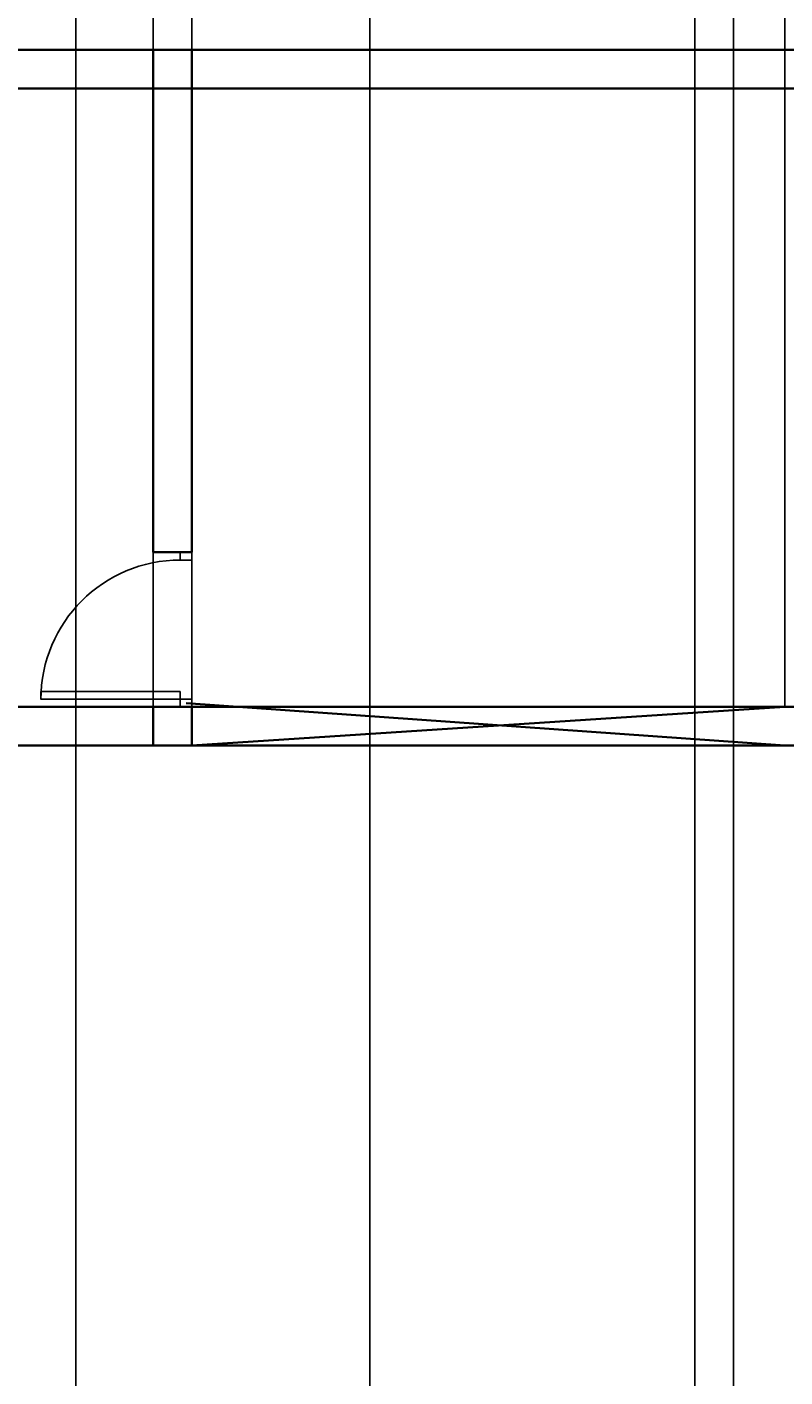
# Model space of a CAD drawing. Units: inches. Extents: x 867 to 1667, y -234 to 788.
# Tile 29 of 42: x 1219 to 1395, y 258 to 572. Entities that reach past the tile are written whole.
import ezdxf

# ---------------------------------------------------------------- set-up
doc = ezdxf.new("R2010")
doc.units = ezdxf.units.IN
doc.header["$MEASUREMENT"] = 0
for name, color, linetype, lineweight in [('A-ANNO-DIMS', 2, 'Continuous', 18), ('A-Door', 150, 'Continuous', 25), ('A-Wall', 7, 'Continuous', 35)]:
    doc.layers.add(name, color=color, linetype=linetype, lineweight=lineweight)
doc.layers.add('NET 01', color=8, linetype='Continuous')
doc.styles.get("Standard").update_dxf_attribs({"font": 'arial.ttf'})
doc.dimstyles.get("Standard").update_dxf_attribs({"dimtxt": 0.6875, "dimasz": 0.18, "dimexe": 0.18, "dimexo": 0.0625, "dimgap": 0.09, "dimtad": 0, "dimdec": 4, "dimzin": 0, "dimdsep": 46, "dimlunit": 4, "dimtxsty": 'Standard', "dimcen": 0.09, "dimadec": 0, "dimazin": 0, "dimtfac": 1, "dimtdec": 4, "dimtofl": 0, "dimtmove": 0, "dimatfit": 3, "dimfxl": 1, "dimtolj": 1, "dimtzin": 0, "dimarcsym": 0})

# ---------------------------------------------------------------- blocks, each defined once
blk = doc.blocks.new('A$C292B336C')
at = {"layer": 'A-Door'}
for points in [[(-0.05, 0), (-0.05, 0.9), (0, 0.9), (0, 0)], [(-0.95, 0), (-0.95, -0.075), (-0.9, -0.075), (-0.9, 0)], [(0, 0), (0, -0.075), (0.05, -0.075), (0.05, 0)]]:
    blk.add_lwpolyline(points, close=True, dxfattribs=at)
at = {"layer": 'NET 01'}
blk.add_arc((0, 0), 0.9, 90, 180, dxfattribs=at)
blk = doc.blocks.new('*D23')
at = {"layer": 'A-ANNO-DIMS', "color": 0, "lineweight": -2, "transparency": 16777216}
for p, q in [((1373.89, 623.55), (1373.89, -233.54)), ((1382.89, 623.55), (1382.89, -233.54)), ((1374.07, -233.36), (1378.07, -233.36)), ((1382.71, -233.36), (1378.7, -233.36))]:
    blk.add_line(p, q, dxfattribs=at)
at = {"layer": 'A-ANNO-DIMS', "color": 0, "transparency": 16777216}
for points in [[(1374.07, -233.33), (1374.07, -233.39), (1373.89, -233.36)], [(1382.71, -233.33), (1382.71, -233.39), (1382.89, -233.36)]]:
    blk.add_solid(points, dxfattribs=at)
at = {"layer": 'Defpoints', "color": 0, "transparency": 16777216}
for p in [(1373.89, 623.62), (1382.89, 623.62), (1382.89, -233.36)]:
    blk.add_point(p, dxfattribs=at)
at = {"layer": 'A-ANNO-DIMS', "color": 0, "transparency": 16777216, "insert": (1378.39, -233.36), "char_height": 0.688, "attachment_point": 5}
blk.add_mtext('\\A1;9', dxfattribs=at)
blk = doc.blocks.new('*D30')
at = {"layer": 'A-ANNO-DIMS', "color": 0, "lineweight": -2, "transparency": 16777216}
for p, q in [((1229.89, 623.55), (1229.89, -233.54)), ((1298.3, 623.55), (1298.3, -233.54)), ((1230.07, -233.36), (1262.91, -233.36)), ((1298.12, -233.36), (1265.28, -233.36))]:
    blk.add_line(p, q, dxfattribs=at)
at = {"layer": 'A-ANNO-DIMS', "color": 0, "transparency": 16777216}
for points in [[(1230.07, -233.33), (1230.07, -233.39), (1229.89, -233.36)], [(1298.12, -233.33), (1298.12, -233.39), (1298.3, -233.36)]]:
    blk.add_solid(points, dxfattribs=at)
at = {"layer": 'Defpoints', "color": 0, "transparency": 16777216}
for p in [(1229.89, 623.62), (1298.3, 623.62), (1298.3, -233.36)]:
    blk.add_point(p, dxfattribs=at)
at = {"layer": 'A-ANNO-DIMS', "color": 0, "transparency": 16777216, "insert": (1264.09, -233.36), "char_height": 0.688, "attachment_point": 5}
blk.add_mtext('\\A1;68.41', dxfattribs=at)
blk = doc.blocks.new('*D31')
at = {"layer": 'A-ANNO-DIMS', "color": 0, "lineweight": -2, "transparency": 16777216}
for p, q in [((1070.89, 566.68), (1070.89, 787.75)), ((1071.07, 787.57), (1304.02, 787.57)), ((1538.71, 787.57), (1305.75, 787.57)), ((1538.89, 566.68), (1538.89, 787.75))]:
    blk.add_line(p, q, dxfattribs=at)
at = {"layer": 'A-ANNO-DIMS', "color": 0, "transparency": 16777216}
for points in [[(1071.07, 787.6), (1071.07, 787.54), (1070.89, 787.57)], [(1538.71, 787.6), (1538.71, 787.54), (1538.89, 787.57)]]:
    blk.add_solid(points, dxfattribs=at)
at = {"layer": 'Defpoints', "color": 0, "transparency": 16777216}
for p in [(1538.89, 787.57), (1070.89, 566.62), (1538.89, 566.62)]:
    blk.add_point(p, dxfattribs=at)
at = {"layer": 'A-ANNO-DIMS', "color": 0, "transparency": 16777216, "insert": (1304.89, 787.57), "char_height": 0.688, "attachment_point": 5}
blk.add_mtext('\\A1;468', dxfattribs=at)
blk = doc.blocks.new('*D32')
at = {"layer": 'A-ANNO-DIMS', "color": 0, "lineweight": -2, "transparency": 16777216}
for p, q in [((1079.89, 404.68), (1079.89, 787.75)), ((1080.07, 787.57), (1163.07, 787.57)), ((1247.71, 787.57), (1164.7, 787.57)), ((1247.89, 413.68), (1247.89, 787.75))]:
    blk.add_line(p, q, dxfattribs=at)
at = {"layer": 'A-ANNO-DIMS', "color": 0, "transparency": 16777216}
for points in [[(1080.07, 787.6), (1080.07, 787.54), (1079.89, 787.57)], [(1247.71, 787.6), (1247.71, 787.54), (1247.89, 787.57)]]:
    blk.add_solid(points, dxfattribs=at)
at = {"layer": 'Defpoints', "color": 0, "transparency": 16777216}
for p in [(1247.89, 787.57), (1247.89, 413.62), (1079.89, 404.62)]:
    blk.add_point(p, dxfattribs=at)
at = {"layer": 'A-ANNO-DIMS', "color": 0, "transparency": 16777216, "insert": (1163.89, 787.57), "char_height": 0.688, "attachment_point": 5}
blk.add_mtext('\\A1;168', dxfattribs=at)
blk = doc.blocks.new('*D33')
at = {"layer": 'A-ANNO-DIMS', "color": 0, "lineweight": -2, "transparency": 16777216}
for p, q in [((1256.89, 413.68), (1256.89, 787.75)), ((1257.07, 787.57), (1325.07, 787.57)), ((1394.71, 787.57), (1326.7, 787.57)), ((1394.89, 413.68), (1394.89, 787.75))]:
    blk.add_line(p, q, dxfattribs=at)
at = {"layer": 'A-ANNO-DIMS', "color": 0, "transparency": 16777216}
for points in [[(1257.07, 787.6), (1257.07, 787.54), (1256.89, 787.57)], [(1394.71, 787.6), (1394.71, 787.54), (1394.89, 787.57)]]:
    blk.add_solid(points, dxfattribs=at)
at = {"layer": 'Defpoints', "color": 0, "transparency": 16777216}
for p in [(1394.89, 787.57), (1256.89, 413.62), (1394.89, 413.62)]:
    blk.add_point(p, dxfattribs=at)
at = {"layer": 'A-ANNO-DIMS', "color": 0, "transparency": 16777216, "insert": (1325.89, 787.57), "char_height": 0.688, "attachment_point": 5}
blk.add_mtext('\\A1;138', dxfattribs=at)

msp = doc.modelspace()

# ---------------------------------------------------------------- linework, layer by layer
at = {"layer": 'A-Wall'}
for p, q in [((1538.8866, 566.617), (1070.8866, 566.617)), ((1247.8866, 566.617), (1247.8866, 449.617)), ((1256.8866, 566.617), (1256.8866, 449.617)), ((1538.8866, 557.617), (1070.8866, 557.617)), ((1247.8866, 449.617), (1256.8866, 449.617)), ((1529.8866, 413.617), (1040.8866, 413.617)), ((1247.8866, 413.617), (1247.8866, 404.617)), ((1255.5362, 414.5056), (1394.8866, 404.617)), ((1256.8866, 413.617), (1256.8866, 404.617)), ((1394.8866, 413.617), (1256.8866, 404.617)), ((1559.8866, 404.617), (1040.8866, 404.617))]:
    msp.add_line(p, q, dxfattribs=at)

# ---------------------------------------------------------------- block references
at = {"layer": 'A-Door', "xscale": -36.01171521992244, "yscale": 36.01171521992244, "zscale": 36.01171521992244, "rotation": 90}
msp.add_blockref('A$C292B336C', (1254.1857, 415.4059), dxfattribs=at)

# ---------------------------------------------------------------- dimensions: what is measured, and where the dimension line sits
at = {"layer": 'A-ANNO-DIMS'}
for base, p1, p2, override, picture, middle in [((1538.8866, 787.567), (1070.8866, 566.617), (1538.8866, 566.617), {"dimdec": 0, "dimlfac": 1, "dimrnd": 0, "dimzin": 0, "dimdsep": 46, "dimlunit": 2}, '*D31', (1304.8866, 787.567)), ((1247.8866, 787.567), (1079.8866, 404.617), (1247.8866, 413.617), {"dimdec": 0, "dimlfac": 1, "dimrnd": 0, "dimzin": 0, "dimdsep": 46, "dimlunit": 2}, '*D32', (1163.8866, 787.567)), ((1394.8866, 787.567), (1256.8866, 413.617), (1394.8866, 413.617), {"dimdec": 0, "dimlfac": 1, "dimrnd": 0, "dimzin": 0, "dimdsep": 46, "dimlunit": 2}, '*D33', (1325.8866, 787.567)), ((1298.2966, -233.3581), (1229.8866, 623.617), (1298.2966, 623.617), {"dimdec": 2, "dimlfac": 1, "dimrnd": 0, "dimzin": 0, "dimdsep": 46, "dimlunit": 2}, '*D30', (1264.0916, -233.3581)), ((1382.8866, -233.3581), (1373.8866, 623.617), (1382.8866, 623.617), {"dimdec": 0, "dimlfac": 1, "dimrnd": 0, "dimzin": 0, "dimdsep": 46, "dimlunit": 2}, '*D23', (1378.3866, -233.3581))]:
    dim = msp.add_linear_dim(base=base, p1=p1, p2=p2, dimstyle='Standard', override=override, dxfattribs=at)
    dim.commit()
    dim.dimension.update_dxf_attribs({"geometry": picture, "text_midpoint": middle})

doc.saveas('drawing.dxf')
